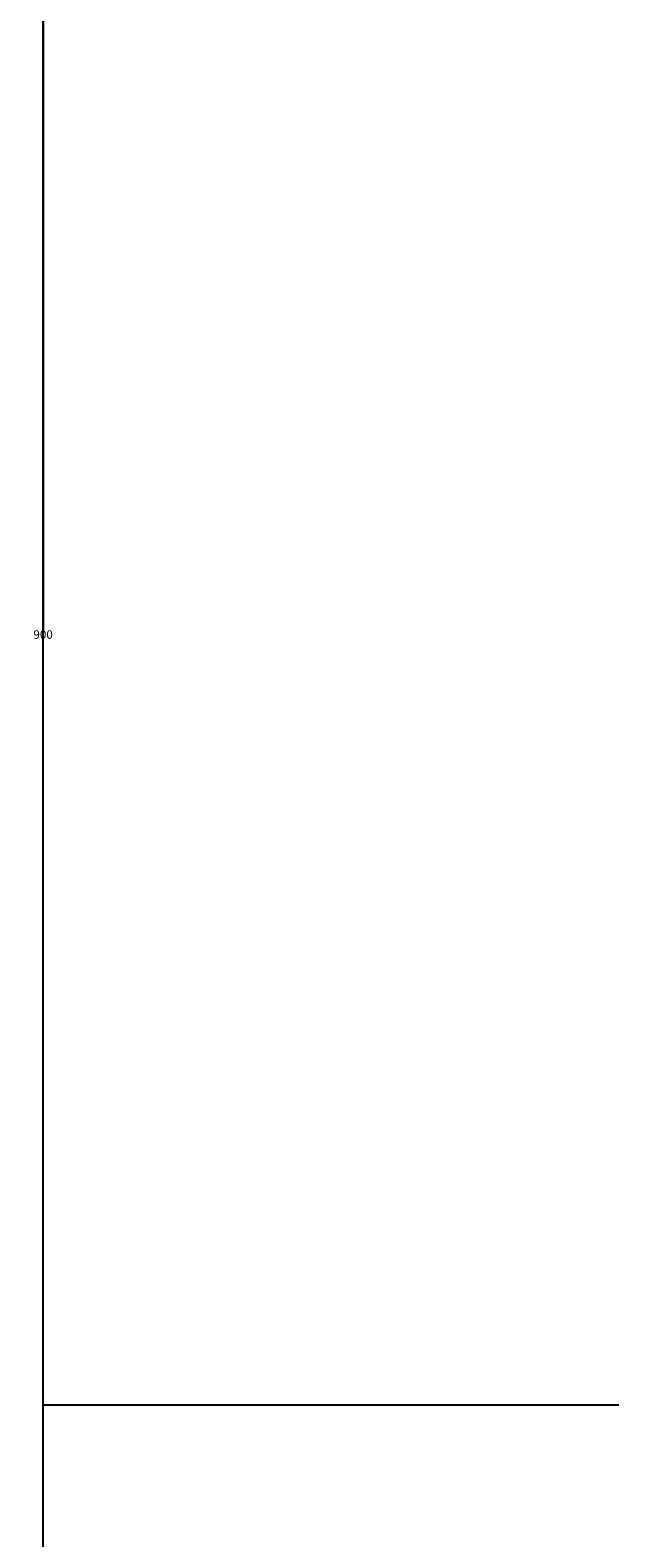
# Model space of a CAD drawing. Units: metres. Extents: x -2391 to 4922, y -635 to 4845.
# Tile 3 of 37: x -2391 to -2049, y 528 to 1408. Entities that reach past the tile are written whole.
import ezdxf

# ---------------------------------------------------------------- set-up
doc = ezdxf.new("R2010")
doc.units = ezdxf.units.M
doc.header["$MEASUREMENT"] = 0
doc.layers.add('A-ANNO-DIMS', color=2, linetype='Continuous', lineweight=18)
doc.styles.get("Standard").update_dxf_attribs({"font": 'arial.ttf'})
doc.dimstyles.get("Standard").update_dxf_attribs({"dimtxt": 5, "dimasz": 4, "dimexe": 0.18, "dimexo": 0.0625, "dimgap": 0.09, "dimtad": 0, "dimtih": 1, "dimtoh": 1, "dimdec": 0, "dimzin": 0, "dimdsep": 46, "dimtxsty": 'Standard', "dimcen": 0.09, "dimadec": 0, "dimazin": 0, "dimtfac": 1, "dimtdec": 0, "dimtofl": 0, "dimtmove": 0, "dimatfit": 3, "dimfxl": 1, "dimtolj": 1, "dimtzin": 0, "dimarcsym": 0})

# ---------------------------------------------------------------- blocks, each defined once
blk = doc.blocks.new('*D10')
at = {"layer": 'A-ANNO-DIMS', "color": 0, "lineweight": -2, "transparency": 16777216}
for p, q in [((550.68, 4505.28), (-2384.01, 4505.28)), ((-2383.83, 4501.28), (-2383.83, 2107.92)), ((-2383.83, -290.72), (-2383.83, 2102.63)), ((-488.55, -294.72), (-2384.01, -294.72))]:
    blk.add_line(p, q, dxfattribs=at)
at = {"layer": 'A-ANNO-DIMS', "color": 0, "transparency": 16777216}
for points in [[(-2384.5, 4501.28), (-2383.17, 4501.28), (-2383.83, 4505.28)], [(-2384.5, -290.72), (-2383.17, -290.72), (-2383.83, -294.72)]]:
    blk.add_solid(points, dxfattribs=at)
at = {"layer": 'Defpoints', "color": 0, "transparency": 16777216}
for p in [(-2383.83, 4505.28), (550.74, 4505.28), (-488.49, -294.72)]:
    blk.add_point(p, dxfattribs=at)
at = {"layer": 'A-ANNO-DIMS', "color": 0, "transparency": 16777216, "insert": (-2383.83, 2105.28), "char_height": 5, "attachment_point": 5}
blk.add_mtext('\\A1;4800', dxfattribs=at)
blk = doc.blocks.new('*D44')
at = {"layer": 'A-ANNO-DIMS', "color": 0, "lineweight": -2, "transparency": 16777216}
for p, q in [((-2047.4, 1505.28), (-2384.01, 1505.28)), ((-2383.83, 1501.28), (-2383.83, 1057.92)), ((-2383.83, 609.28), (-2383.83, 1052.63)), ((-2047.4, 605.28), (-2384.01, 605.28))]:
    blk.add_line(p, q, dxfattribs=at)
at = {"layer": 'A-ANNO-DIMS', "color": 0, "transparency": 16777216}
for points in [[(-2384.5, 1501.28), (-2383.17, 1501.28), (-2383.83, 1505.28)], [(-2384.5, 609.28), (-2383.17, 609.28), (-2383.83, 605.28)]]:
    blk.add_solid(points, dxfattribs=at)
at = {"layer": 'Defpoints', "color": 0, "transparency": 16777216}
for p in [(-2047.33, 1505.28), (-2383.83, 605.28), (-2047.33, 605.28)]:
    blk.add_point(p, dxfattribs=at)
at = {"layer": 'A-ANNO-DIMS', "color": 0, "transparency": 16777216, "insert": (-2383.83, 1055.28), "char_height": 5, "attachment_point": 5}
blk.add_mtext('\\A1;900', dxfattribs=at)

msp = doc.modelspace()

# ---------------------------------------------------------------- dimensions: what is measured, and where the dimension line sits
at = {"layer": 'A-ANNO-DIMS'}
for base, p1, p2, picture, middle in [((-2383.8343, 4505.2763), (-488.4886, -294.7237), (550.7419, 4505.2763), '*D10', (-2383.8343, 2105.2763)), ((-2383.8343, 605.2763), (-2047.3343, 1505.2763), (-2047.3343, 605.2763), '*D44', (-2383.8343, 1055.2763))]:
    dim = msp.add_linear_dim(base=base, p1=p1, p2=p2, angle=90, dimstyle='Standard', override={"dimdec": 0, "dimlfac": 1, "dimrnd": 0, "dimzin": 0, "dimdsep": 46, "dimlunit": 2}, dxfattribs=at)
    dim.commit()
    dim.dimension.update_dxf_attribs({"geometry": picture, "text_midpoint": middle})

doc.saveas('drawing.dxf')
